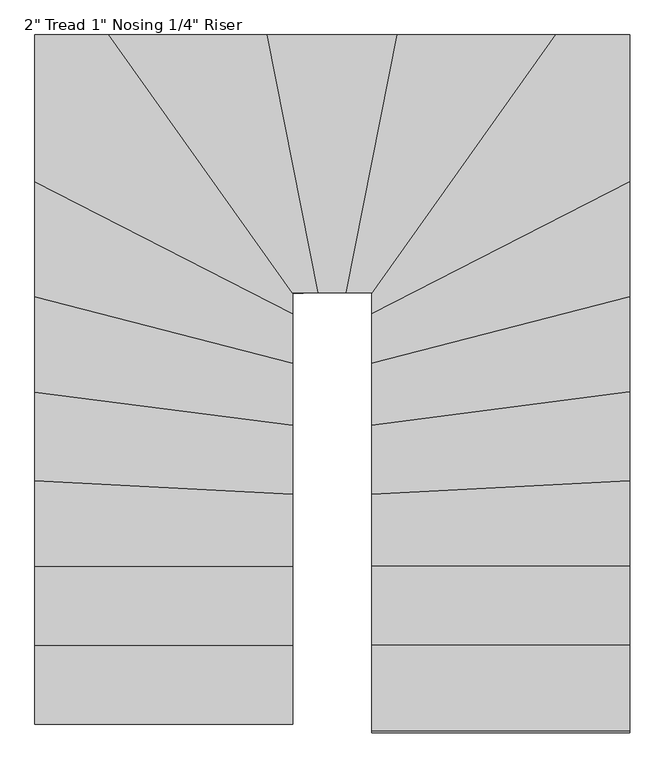
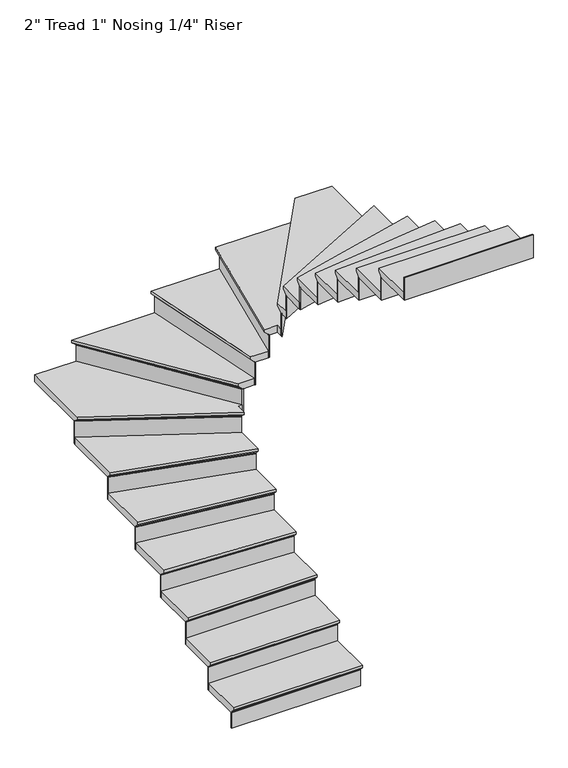
"""IFC4 building model written with IfcOpenShell, lengths in millimetres: stair flight geometry."""

from ifc_helpers import new_model, si_unit, origin, place, context, project, spatial, faceted_brep, source, transform, mapped, element, save


def stair_flight_9737d4c8(model_context):
    return source(origin(), model_context, "Body", "Brep", [
        faceted_brep([(-715.0890964, 3647.9718401, 6551.0833333), (-715.0890964, 3647.9718401, 6570.1333333), (-1629.4890964, 3647.9718401, 6570.1333333), (-1629.4890964, 3647.9718401, 6551.0833333), (-715.0890964, 3673.3718401, 6525.6833333), (-1629.4890964, 3673.3718401, 6525.6833333), (-715.0890964, 3952.7718401, 6570.1333333), (-1629.4890964, 3952.7718401, 6570.1333333), (-1629.4890964, 3673.3718401, 6519.3333333), (-1629.4890964, 3952.7718401, 6519.3333333), (-715.0890964, 3952.7718401, 6519.3333333), (-715.0890964, 3673.3718401, 6519.3333333)], [[[0, 1, 2, 3]], [[4, 0, 3, 5]], [[2, 1, 6, 7]], [[8, 9, 10, 11]], [[2, 7, 9, 8, 5, 3]], [[8, 11, 4, 5]], [[6, 1, 0, 4, 11, 10]], [[7, 6, 10, 9]]]),
        faceted_brep([(-715.0890964, 3673.3718401, 6519.3333333), (-715.0890964, 3673.3718401, 6400.8), (-715.0890964, 3679.7218401, 6400.8), (-715.0890964, 3679.7218401, 6519.3333333), (-1629.4890964, 3673.3718401, 6519.3333333), (-1629.4890964, 3679.7218401, 6519.3333333), (-1629.4890964, 3679.7218401, 6400.8), (-1629.4890964, 3673.3718401, 6400.8)], [[[0, 1, 2, 3]], [[4, 5, 6, 7]], [[1, 0, 4, 7]], [[2, 1, 7, 6]], [[3, 2, 6, 5]], [[0, 3, 5, 4]]]),
        faceted_brep([(-715.0890964, 3952.7718401, 6688.6666667), (-715.0890964, 3952.7718401, 6519.3333333), (-715.0890964, 3959.1218401, 6519.3333333), (-715.0890964, 3959.1218401, 6688.6666667), (-1629.4890964, 3952.7718401, 6688.6666667), (-1629.4890964, 3959.1218401, 6688.6666667), (-1629.4890964, 3959.1218401, 6519.3333333), (-1629.4890964, 3952.7718401, 6519.3333333)], [[[0, 1, 2, 3]], [[4, 5, 6, 7]], [[1, 0, 4, 7]], [[2, 1, 7, 6]], [[3, 2, 6, 5]], [[0, 3, 5, 4]]]),
        faceted_brep([(-1629.4890964, 3927.3718401, 6739.4666667), (-715.0890964, 3927.3718401, 6739.4666667), (-715.0890964, 4232.1718401, 6739.4666667), (-1629.4890964, 4232.1718401, 6739.4666667), (-1629.4890964, 3952.7718401, 6688.6666667), (-1629.4890964, 4232.1718401, 6688.6666667), (-715.0890964, 4232.1718401, 6688.6666667), (-715.0890964, 3952.7718401, 6688.6666667), (-1629.4890964, 3952.7718401, 6695.0166667), (-1629.4890964, 3927.3718401, 6720.4166667), (-715.0890964, 3952.7718401, 6695.0166667), (-715.0890964, 3927.3718401, 6720.4166667)], [[[0, 1, 2, 3]], [[4, 5, 6, 7]], [[0, 3, 5, 4, 8, 9]], [[4, 7, 10, 8]], [[2, 1, 11, 10, 7, 6]], [[3, 2, 6, 5]], [[11, 1, 0, 9]], [[10, 11, 9, 8]]]),
        faceted_brep([(-715.0890964, 4232.1718401, 6858.0), (-715.0890964, 4232.1718401, 6688.6666667), (-715.0890964, 4238.5218401, 6688.6666667), (-715.0890964, 4238.5218401, 6858.0), (-1629.4890964, 4232.1718401, 6858.0), (-1629.4890964, 4238.5218401, 6858.0), (-1629.4890964, 4238.5218401, 6688.6666667), (-1629.4890964, 4232.1718401, 6688.6666667)], [[[0, 1, 2, 3]], [[4, 5, 6, 7]], [[1, 0, 4, 7]], [[2, 1, 7, 6]], [[3, 2, 6, 5]], [[0, 3, 5, 4]]]),
        faceted_brep([(-1629.4890964, 4206.7718401, 6908.8), (-715.0890964, 4206.7718401, 6908.8), (-715.0890964, 4487.8390016, 6908.8), (-1629.4890964, 4535.373272, 6908.8), (-1629.4890964, 4232.1718401, 6858.0), (-1629.4890964, 4535.373272, 6858.0), (-715.0890964, 4487.8390016, 6858.0), (-715.0890964, 4232.1718401, 6858.0), (-1629.4890964, 4232.1718401, 6864.35), (-1629.4890964, 4206.7718401, 6889.75), (-715.0890964, 4232.1718401, 6864.35), (-715.0890964, 4206.7718401, 6889.75)], [[[0, 1, 2, 3]], [[4, 5, 6, 7]], [[0, 3, 5, 4, 8, 9]], [[4, 7, 10, 8]], [[2, 1, 11, 10, 7, 6]], [[3, 2, 6, 5]], [[11, 1, 0, 9]], [[10, 11, 9, 8]]]),
        faceted_brep([(-715.0890964, 4487.8390016, 7027.3333333), (-715.0890964, 4487.8390016, 6858.0), (-715.0890964, 4494.1975757, 6858.0), (-715.0890964, 4494.1975757, 7027.3333333), (-1629.4890964, 4535.373272, 7027.3333333), (-1629.4890964, 4541.7318461, 7027.3333333), (-1629.4890964, 4541.7318461, 6858.0), (-1629.4890964, 4535.373272, 6858.0)], [[[0, 1, 2, 3]], [[4, 5, 6, 7]], [[1, 0, 4, 7]], [[2, 1, 7, 6]], [[3, 2, 6, 5]], [[0, 3, 5, 4]]]),
        faceted_brep([(-1629.4890964, 4509.9389753, 7078.1333333), (-715.0890964, 4462.4047049, 7078.1333333), (-715.0890964, 4732.0057014, 7078.1333333), (-1629.4890964, 4850.361753, 7078.1333333), (-1629.4890964, 4535.373272, 7027.3333333), (-1629.4890964, 4850.361753, 7027.3333333), (-715.0890964, 4732.0057014, 7027.3333333), (-715.0890964, 4487.8390016, 7027.3333333), (-1629.4890964, 4535.373272, 7033.6833333), (-1629.4890964, 4509.9389753, 7059.0833333), (-715.0890964, 4487.8390016, 7033.6833333), (-715.0890964, 4462.4047049, 7059.0833333)], [[[0, 1, 2, 3]], [[4, 5, 6, 7]], [[0, 3, 5, 4, 8, 9]], [[4, 7, 10, 8]], [[2, 1, 11, 10, 7, 6]], [[3, 2, 6, 5]], [[11, 1, 0, 9]], [[10, 11, 9, 8]]]),
        faceted_brep([(-715.0890964, 4732.0057014, 7196.6666667), (-715.0890964, 4732.0057014, 7027.3333333), (-715.0890964, 4738.4086732, 7027.3333333), (-715.0890964, 4738.4086732, 7196.6666667), (-1629.4890964, 4850.361753, 7196.6666667), (-1629.4890964, 4856.7647248, 7196.6666667), (-1629.4890964, 4856.7647248, 7027.3333333), (-1629.4890964, 4850.361753, 7027.3333333)], [[[0, 1, 2, 3]], [[4, 5, 6, 7]], [[1, 0, 4, 7]], [[2, 1, 7, 6]], [[3, 2, 6, 5]], [[0, 3, 5, 4]]]),
        faceted_brep([(-1629.4890964, 4824.7498659, 7247.4666667), (-715.0890964, 4706.3938143, 7247.4666667), (-715.0890964, 4953.6329239, 7247.4666667), (-1629.4890964, 5188.7633713, 7247.4666667), (-1629.4890964, 4850.361753, 7196.6666667), (-1629.4890964, 5188.7633713, 7196.6666667), (-715.0890964, 4953.6329239, 7196.6666667), (-715.0890964, 4732.0057014, 7196.6666667), (-1629.4890964, 4850.361753, 7203.0166667), (-1629.4890964, 4824.7498659, 7228.4166667), (-715.0890964, 4732.0057014, 7203.0166667), (-715.0890964, 4706.3938143, 7228.4166667)], [[[0, 1, 2, 3]], [[4, 5, 6, 7]], [[0, 3, 5, 4, 8, 9]], [[4, 7, 10, 8]], [[2, 1, 11, 10, 7, 6]], [[3, 2, 6, 5]], [[11, 1, 0, 9]], [[10, 11, 9, 8]]]),
        faceted_brep([(-715.0890964, 4953.6329239, 7366.0), (-715.0890964, 4953.6329239, 7196.6666667), (-715.0890964, 4960.1895007, 7196.6666667), (-715.0890964, 4960.1895007, 7366.0), (-1629.4890964, 5188.7633713, 7366.0), (-1629.4890964, 5195.3199481, 7366.0), (-1629.4890964, 5195.3199481, 7196.6666667), (-1629.4890964, 5188.7633713, 7196.6666667)], [[[0, 1, 2, 3]], [[4, 5, 6, 7]], [[1, 0, 4, 7]], [[2, 1, 7, 6]], [[3, 2, 6, 5]], [[0, 3, 5, 4]]]),
        faceted_brep([(-1629.4890964, 5162.5370638, 7416.8), (-715.0890964, 4927.4066164, 7416.8), (-715.0890964, 5129.9795599, 7416.8), (-1629.4890964, 5598.8041813, 7416.8), (-1629.4890964, 5188.7633713, 7366.0), (-1629.4890964, 5598.8041813, 7366.0), (-715.0890964, 5129.9795599, 7366.0), (-715.0890964, 4953.6329239, 7366.0), (-1629.4890964, 5188.7633713, 7372.35), (-1629.4890964, 5162.5370638, 7397.75), (-715.0890964, 4953.6329239, 7372.35), (-715.0890964, 4927.4066164, 7397.75)], [[[0, 1, 2, 3]], [[4, 5, 6, 7]], [[0, 3, 5, 4, 8, 9]], [[4, 7, 10, 8]], [[2, 1, 11, 10, 7, 6]], [[3, 2, 6, 5]], [[11, 1, 0, 9]], [[10, 11, 9, 8]]]),
        faceted_brep([(-715.0890964, 5129.9795599, 7535.3333333), (-715.0890964, 5129.9795599, 7366.0), (-715.0890964, 5137.1155431, 7366.0), (-715.0890964, 5137.1155431, 7535.3333333), (-1629.4890964, 5598.8041813, 7535.3333333), (-1629.4890964, 5605.9401644, 7535.3333333), (-1629.4890964, 5605.9401644, 7366.0), (-1629.4890964, 5598.8041813, 7366.0)], [[[0, 1, 2, 3]], [[4, 5, 6, 7]], [[1, 0, 4, 7]], [[2, 1, 7, 6]], [[3, 2, 6, 5]], [[0, 3, 5, 4]]]),
        faceted_brep([(-1335.8079627, 6090.103532, 7586.1333333), (-1629.4890964, 6090.103532, 7586.1333333), (-1629.4890964, 5570.2602487, 7586.1333333), (-715.0890964, 5101.4356274, 7586.1333333), (-715.0890964, 5175.703532, 7586.1333333), (-685.5340135, 5175.703532, 7586.1333333), (-1629.4890964, 6090.103532, 7535.3333333), (-1335.8079627, 6090.103532, 7535.3333333), (-685.5340135, 5175.703532, 7535.3333333), (-715.0890964, 5175.703532, 7535.3333333), (-715.0890964, 5129.9795599, 7535.3333333), (-1629.4890964, 5598.8041813, 7535.3333333), (-1629.4890964, 5598.8041813, 7541.6833333), (-1629.4890964, 5570.2602487, 7567.0833333), (-715.0890964, 5129.9795599, 7541.6833333), (-715.0890964, 5101.4356274, 7567.0833333)], [[[0, 1, 2, 3, 4, 5]], [[6, 7, 8, 9, 10, 11]], [[1, 0, 7, 6]], [[2, 1, 6, 11, 12, 13]], [[11, 10, 14, 12]], [[4, 3, 15, 14, 10, 9]], [[5, 4, 9, 8]], [[0, 5, 8, 7]], [[15, 3, 2, 13]], [[14, 15, 13, 12]]]),
        faceted_brep([(-685.5340135, 5175.703532, 7704.6666667), (-685.5340135, 5175.703532, 7535.3333333), (-677.7420387, 5175.703532, 7535.3333333), (-677.7420387, 5175.703532, 7704.6666667), (-1335.8079627, 6090.103532, 7704.6666667), (-1328.0159879, 6090.103532, 7704.6666667), (-1328.0159879, 6090.103532, 7535.3333333), (-1335.8079627, 6090.103532, 7535.3333333)], [[[0, 1, 2, 3]], [[4, 5, 6, 7]], [[1, 0, 4, 7]], [[2, 1, 7, 6]], [[3, 2, 6, 5]], [[0, 3, 5, 4]]]),
        faceted_brep([(-1366.9758618, 6090.103532, 7755.4666667), (-716.7019127, 5175.703532, 7755.4666667), (-599.0799265, 5175.703532, 7755.4666667), (-779.3207828, 6090.103532, 7755.4666667), (-1335.8079627, 6090.103532, 7704.6666667), (-779.3207828, 6090.103532, 7704.6666667), (-599.0799265, 5175.703532, 7704.6666667), (-685.5340135, 5175.703532, 7704.6666667), (-1335.8079627, 6090.103532, 7711.0166667), (-1366.9758618, 6090.103532, 7736.4166667), (-685.5340135, 5175.703532, 7711.0166667), (-716.7019127, 5175.703532, 7736.4166667)], [[[0, 1, 2, 3]], [[4, 5, 6, 7]], [[0, 3, 5, 4, 8, 9]], [[4, 7, 10, 8]], [[2, 1, 11, 10, 7, 6]], [[3, 2, 6, 5]], [[11, 1, 0, 9]], [[10, 11, 9, 8]]]),
        faceted_brep([(-599.0799265, 5175.703532, 7874.0), (-599.0799265, 5175.703532, 7704.6666667), (-592.607741, 5175.703532, 7704.6666667), (-592.607741, 5175.703532, 7874.0), (-779.3207828, 6090.103532, 7874.0), (-772.8485973, 6090.103532, 7874.0), (-772.8485973, 6090.103532, 7704.6666667), (-779.3207828, 6090.103532, 7704.6666667)], [[[0, 1, 2, 3]], [[4, 5, 6, 7]], [[1, 0, 4, 7]], [[2, 1, 7, 6]], [[3, 2, 6, 5]], [[0, 3, 5, 4]]]),
        faceted_brep([(-805.2095245, 6090.103532, 7924.8), (-624.9686682, 5175.703532, 7924.8), (-499.9207828, 5175.703532, 7924.8), (-319.6799265, 6090.103532, 7924.8), (-779.3207828, 6090.103532, 7874.0), (-319.6799265, 6090.103532, 7874.0), (-499.9207828, 5175.703532, 7874.0), (-599.0799265, 5175.703532, 7874.0), (-779.3207828, 6090.103532, 7880.35), (-805.2095245, 6090.103532, 7905.75), (-599.0799265, 5175.703532, 7880.35), (-624.9686682, 5175.703532, 7905.75)], [[[0, 1, 2, 3]], [[4, 5, 6, 7]], [[0, 3, 5, 4, 8, 9]], [[4, 7, 10, 8]], [[2, 1, 11, 10, 7, 6]], [[3, 2, 6, 5]], [[11, 1, 0, 9]], [[10, 11, 9, 8]]]),
        faceted_brep([(-499.9207828, 5175.703532, 8043.3333333), (-499.9207828, 5175.703532, 7874.0), (-493.4485973, 5175.703532, 7874.0), (-493.4485973, 5175.703532, 8043.3333333), (-319.6799265, 6090.103532, 8043.3333333), (-313.207741, 6090.103532, 8043.3333333), (-313.207741, 6090.103532, 7874.0), (-319.6799265, 6090.103532, 7874.0)], [[[0, 1, 2, 3]], [[4, 5, 6, 7]], [[1, 0, 4, 7]], [[2, 1, 7, 6]], [[3, 2, 6, 5]], [[0, 3, 5, 4]]]),
        faceted_brep([(-345.5686682, 6090.103532, 8094.1333333), (-525.8095245, 5175.703532, 8094.1333333), (-435.6890964, 5175.703532, 8094.1333333), (-435.6890964, 5129.6080574, 8094.1333333), (247.3655683, 6090.103532, 8094.1333333), (-319.6799265, 6090.103532, 8043.3333333), (247.3655683, 6090.103532, 8043.3333333), (-435.6890964, 5129.6080574, 8043.3333333), (-435.6890964, 5175.703532, 8043.3333333), (-499.9207828, 5175.703532, 8043.3333333), (-319.6799265, 6090.103532, 8049.6833333), (-345.5686682, 6090.103532, 8075.0833333), (-499.9207828, 5175.703532, 8049.6833333), (-525.8095245, 5175.703532, 8075.0833333)], [[[0, 1, 2, 3, 4]], [[5, 6, 7, 8, 9]], [[0, 4, 6, 5, 10, 11]], [[5, 9, 12, 10]], [[2, 1, 13, 12, 9, 8]], [[3, 2, 8, 7]], [[4, 3, 7, 6]], [[13, 1, 0, 11]], [[12, 13, 11, 10]]]),
        faceted_brep([(-435.6890964, 5129.6080574, 8212.6666667), (-435.6890964, 5129.6080574, 8043.3333333), (-435.6890964, 5118.6511649, 8043.3333333), (-435.6890964, 5118.6511649, 8212.6666667), (247.3655683, 6090.103532, 8212.6666667), (255.1575431, 6090.103532, 8212.6666667), (255.1575431, 6090.103532, 8043.3333333), (247.3655683, 6090.103532, 8043.3333333)], [[[0, 1, 2, 3]], [[4, 5, 6, 7]], [[1, 0, 4, 7]], [[2, 1, 7, 6]], [[3, 2, 6, 5]], [[0, 3, 5, 4]]]),
        faceted_brep([(478.7109036, 5541.7163162, 8263.4666667), (478.7109036, 6090.103532, 8263.4666667), (216.1976691, 6090.103532, 8263.4666667), (-435.6890964, 5173.4356274, 8263.4666667), (-435.6890964, 5072.8916949, 8263.4666667), (478.7109036, 6090.103532, 8212.6666667), (478.7109036, 5541.7163162, 8212.6666667), (-435.6890964, 5072.8916949, 8212.6666667), (-435.6890964, 5129.6080574, 8212.6666667), (247.3655683, 6090.103532, 8212.6666667), (247.3655683, 6090.103532, 8219.0166667), (216.1976691, 6090.103532, 8244.4166667), (-435.6890964, 5129.6080574, 8219.0166667), (-435.6890964, 5173.4356274, 8244.4166667)], [[[0, 1, 2, 3, 4]], [[5, 6, 7, 8, 9]], [[1, 0, 6, 5]], [[2, 1, 5, 9, 10, 11]], [[9, 8, 12, 10]], [[4, 3, 13, 12, 8, 7]], [[0, 4, 7, 6]], [[13, 3, 2, 11]], [[12, 13, 11, 10]]]),
        faceted_brep([(-435.6890964, 5072.8916949, 8382.0), (-435.6890964, 5072.8916949, 8212.6666667), (-435.6890964, 5065.7557117, 8212.6666667), (-435.6890964, 5065.7557117, 8382.0), (478.7109036, 5541.7163162, 8382.0), (478.7109036, 5534.5803331, 8382.0), (478.7109036, 5534.5803331, 8212.6666667), (478.7109036, 5541.7163162, 8212.6666667)], [[[0, 1, 2, 3]], [[4, 5, 6, 7]], [[1, 0, 4, 7]], [[2, 1, 7, 6]], [[3, 2, 6, 5]], [[0, 3, 5, 4]]]),
        faceted_brep([(478.7109036, 5570.2602487, 8432.8), (-435.6890964, 5101.4356274, 8432.8), (-435.6890964, 4901.1803089, 8432.8), (478.7109036, 5136.3107563, 8432.8), (478.7109036, 5541.7163162, 8382.0), (478.7109036, 5136.3107563, 8382.0), (-435.6890964, 4901.1803089, 8382.0), (-435.6890964, 5072.8916949, 8382.0), (478.7109036, 5541.7163162, 8388.35), (478.7109036, 5570.2602487, 8413.75), (-435.6890964, 5072.8916949, 8388.35), (-435.6890964, 5101.4356274, 8413.75)], [[[0, 1, 2, 3]], [[4, 5, 6, 7]], [[0, 3, 5, 4, 8, 9]], [[4, 7, 10, 8]], [[2, 1, 11, 10, 7, 6]], [[3, 2, 6, 5]], [[11, 1, 0, 9]], [[10, 11, 9, 8]]]),
        faceted_brep([(-435.6890964, 4901.1803089, 8551.3333333), (-435.6890964, 4901.1803089, 8382.0), (-435.6890964, 4894.6237321, 8382.0), (-435.6890964, 4894.6237321, 8551.3333333), (478.7109036, 5136.3107563, 8551.3333333), (478.7109036, 5129.7541795, 8551.3333333), (478.7109036, 5129.7541795, 8382.0), (478.7109036, 5136.3107563, 8382.0)], [[[0, 1, 2, 3]], [[4, 5, 6, 7]], [[1, 0, 4, 7]], [[2, 1, 7, 6]], [[3, 2, 6, 5]], [[0, 3, 5, 4]]]),
        faceted_brep([(478.7109036, 5162.5370638, 8602.1333333), (-435.6890964, 4927.4066164, 8602.1333333), (-435.6890964, 4680.7819272, 8602.1333333), (478.7109036, 4799.1379788, 8602.1333333), (478.7109036, 5136.3107563, 8551.3333333), (478.7109036, 4799.1379788, 8551.3333333), (-435.6890964, 4680.7819272, 8551.3333333), (-435.6890964, 4901.1803089, 8551.3333333), (478.7109036, 5136.3107563, 8557.6833333), (478.7109036, 5162.5370638, 8583.0833333), (-435.6890964, 4901.1803089, 8557.6833333), (-435.6890964, 4927.4066164, 8583.0833333)], [[[0, 1, 2, 3]], [[4, 5, 6, 7]], [[0, 3, 5, 4, 8, 9]], [[4, 7, 10, 8]], [[2, 1, 11, 10, 7, 6]], [[3, 2, 6, 5]], [[11, 1, 0, 9]], [[10, 11, 9, 8]]]),
        faceted_brep([(-435.6890964, 4680.7819272, 8720.6666667), (-435.6890964, 4680.7819272, 8551.3333333), (-435.6890964, 4674.3789554, 8551.3333333), (-435.6890964, 4674.3789554, 8720.6666667), (478.7109036, 4799.1379788, 8720.6666667), (478.7109036, 4792.735007, 8720.6666667), (478.7109036, 4792.735007, 8551.3333333), (478.7109036, 4799.1379788, 8551.3333333)], [[[0, 1, 2, 3]], [[4, 5, 6, 7]], [[1, 0, 4, 7]], [[2, 1, 7, 6]], [[3, 2, 6, 5]], [[0, 3, 5, 4]]]),
        faceted_brep([(478.7109036, 4824.7498659, 8771.4666667), (-435.6890964, 4706.3938143, 8771.4666667), (-435.6890964, 4436.9704082, 8771.4666667), (478.7109036, 4484.5046786, 8771.4666667), (478.7109036, 4799.1379788, 8720.6666667), (478.7109036, 4484.5046786, 8720.6666667), (-435.6890964, 4436.9704082, 8720.6666667), (-435.6890964, 4680.7819272, 8720.6666667), (478.7109036, 4799.1379788, 8727.0166667), (478.7109036, 4824.7498659, 8752.4166667), (-435.6890964, 4680.7819272, 8727.0166667), (-435.6890964, 4706.3938143, 8752.4166667)], [[[0, 1, 2, 3]], [[4, 5, 6, 7]], [[0, 3, 5, 4, 8, 9]], [[4, 7, 10, 8]], [[2, 1, 11, 10, 7, 6]], [[3, 2, 6, 5]], [[11, 1, 0, 9]], [[10, 11, 9, 8]]]),
        faceted_brep([(-435.6890964, 4436.9704082, 8890.0), (-435.6890964, 4436.9704082, 8720.6666667), (-435.6890964, 4430.6118341, 8720.6666667), (-435.6890964, 4430.6118341, 8890.0), (478.7109036, 4484.5046786, 8890.0), (478.7109036, 4478.1461045, 8890.0), (478.7109036, 4478.1461045, 8720.6666667), (478.7109036, 4484.5046786, 8720.6666667)], [[[0, 1, 2, 3]], [[4, 5, 6, 7]], [[1, 0, 4, 7]], [[2, 1, 7, 6]], [[3, 2, 6, 5]], [[0, 3, 5, 4]]]),
        faceted_brep([(478.7109036, 4509.9389753, 8940.8), (-435.6890964, 4462.4047049, 8940.8), (-435.6890964, 4181.3718401, 8940.8), (478.7109036, 4181.3718401, 8940.8), (478.7109036, 4484.5046786, 8890.0), (478.7109036, 4181.3718401, 8890.0), (-435.6890964, 4181.3718401, 8890.0), (-435.6890964, 4436.9704082, 8890.0), (478.7109036, 4484.5046786, 8896.35), (478.7109036, 4509.9389753, 8921.75), (-435.6890964, 4436.9704082, 8896.35), (-435.6890964, 4462.4047049, 8921.75)], [[[0, 1, 2, 3]], [[4, 5, 6, 7]], [[0, 3, 5, 4, 8, 9]], [[4, 7, 10, 8]], [[2, 1, 11, 10, 7, 6]], [[3, 2, 6, 5]], [[11, 1, 0, 9]], [[10, 11, 9, 8]]]),
        faceted_brep([(-435.6890964, 4181.3718401, 9059.3333333), (-435.6890964, 4181.3718401, 8890.0), (-435.6890964, 4175.0218401, 8890.0), (-435.6890964, 4175.0218401, 9059.3333333), (478.7109036, 4181.3718401, 9059.3333333), (478.7109036, 4175.0218401, 9059.3333333), (478.7109036, 4175.0218401, 8890.0), (478.7109036, 4181.3718401, 8890.0)], [[[0, 1, 2, 3]], [[4, 5, 6, 7]], [[1, 0, 4, 7]], [[2, 1, 7, 6]], [[3, 2, 6, 5]], [[0, 3, 5, 4]]]),
        faceted_brep([(478.7109036, 4206.7718401, 9110.1333333), (-435.6890964, 4206.7718401, 9110.1333333), (-435.6890964, 3901.9718401, 9110.1333333), (478.7109036, 3901.9718401, 9110.1333333), (478.7109036, 4181.3718401, 9059.3333333), (478.7109036, 3901.9718401, 9059.3333333), (-435.6890964, 3901.9718401, 9059.3333333), (-435.6890964, 4181.3718401, 9059.3333333), (478.7109036, 4181.3718401, 9065.6833333), (478.7109036, 4206.7718401, 9091.0833333), (-435.6890964, 4181.3718401, 9065.6833333), (-435.6890964, 4206.7718401, 9091.0833333)], [[[0, 1, 2, 3]], [[4, 5, 6, 7]], [[0, 3, 5, 4, 8, 9]], [[4, 7, 10, 8]], [[2, 1, 11, 10, 7, 6]], [[3, 2, 6, 5]], [[11, 1, 0, 9]], [[10, 11, 9, 8]]]),
        faceted_brep([(-435.6890964, 3901.9718401, 9228.6666667), (-435.6890964, 3901.9718401, 9059.3333333), (-435.6890964, 3895.6218401, 9059.3333333), (-435.6890964, 3895.6218401, 9228.6666667), (478.7109036, 3901.9718401, 9228.6666667), (478.7109036, 3895.6218401, 9228.6666667), (478.7109036, 3895.6218401, 9059.3333333), (478.7109036, 3901.9718401, 9059.3333333)], [[[0, 1, 2, 3]], [[4, 5, 6, 7]], [[1, 0, 4, 7]], [[2, 1, 7, 6]], [[3, 2, 6, 5]], [[0, 3, 5, 4]]]),
        faceted_brep([(-435.6890964, 3622.5718401, 9398.0), (-435.6890964, 3622.5718401, 9228.6666667), (-435.6890964, 3616.2218401, 9228.6666667), (-435.6890964, 3616.2218401, 9398.0), (478.7109036, 3622.5718401, 9398.0), (478.7109036, 3616.2218401, 9398.0), (478.7109036, 3616.2218401, 9228.6666667), (478.7109036, 3622.5718401, 9228.6666667)], [[[0, 1, 2, 3]], [[4, 5, 6, 7]], [[1, 0, 4, 7]], [[2, 1, 7, 6]], [[3, 2, 6, 5]], [[0, 3, 5, 4]]]),
        faceted_brep([(478.7109036, 3927.3718401, 9279.4666667), (-435.6890964, 3927.3718401, 9279.4666667), (-435.6890964, 3622.5718401, 9279.4666667), (478.7109036, 3622.5718401, 9279.4666667), (478.7109036, 3901.9718401, 9228.6666667), (478.7109036, 3622.5718401, 9228.6666667), (-435.6890964, 3622.5718401, 9228.6666667), (-435.6890964, 3901.9718401, 9228.6666667), (478.7109036, 3901.9718401, 9235.0166667), (478.7109036, 3927.3718401, 9260.4166667), (-435.6890964, 3901.9718401, 9235.0166667), (-435.6890964, 3927.3718401, 9260.4166667)], [[[0, 1, 2, 3]], [[4, 5, 6, 7]], [[0, 3, 5, 4, 8, 9]], [[4, 7, 10, 8]], [[2, 1, 11, 10, 7, 6]], [[3, 2, 6, 5]], [[11, 1, 0, 9]], [[10, 11, 9, 8]]]),
    ])


if __name__ == "__main__":
    model = new_model("IFC4")
    model_context = context("Model", 3, world=origin())
    ifc_project = project(units=[si_unit("LENGTHUNIT", "METRE", prefix="MILLI")], contexts=[model_context])
    site = spatial("IfcSite", under=ifc_project)
    building = spatial("IfcBuilding", under=site)
    placement = place(None, origin())
    stair_flight_shape = stair_flight_9737d4c8(model_context)
    element("IfcStairFlight", 1, ObjectType="2\" Tread 1\" Nosing 1/4\" Riser", at=placement, inside=building, context=model_context, shape_type="MappedRepresentation", body=[
        mapped(stair_flight_shape, transform((0.0, 0.0, 0.0), x_axis=(1.0, 0.0, 0.0), y_axis=(0.0, 1.0, 0.0), z_axis=(0.0, 0.0, 1.0))),
    ])
    save(model, "model.ifc")
